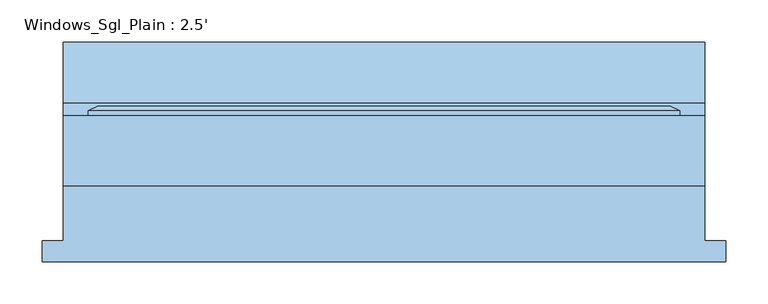
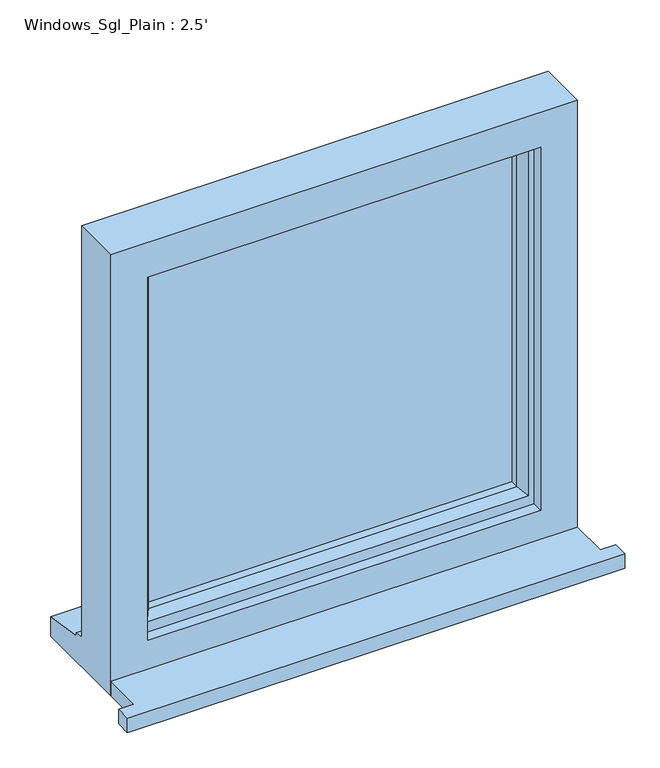
"""IFC4 building model written with IfcOpenShell, lengths in millimetres: window geometry, Windows_Sgl_Plain : 2.5'."""

from ifc_helpers import new_model, si_unit, frame, origin, place, context, project, spatial, polyline, outline, extrude, faceted_brep, source, transform, mapped, element, save


def windows_sgl_plain_2_5_9e76a6e6(model_context):
    return source(origin(), model_context, "Body", "SolidModel", [
        extrude(outline(polyline([(-406.0, -115.6034322), (-406.0, -90.6034322), (-381.0, -90.6034322), (-381.0, -25.4834322), (381.0, -25.4834322), (381.0, -90.6034322), (406.0, -90.6034322), (406.0, -115.6034322), (-406.0, -115.6034322)])), frame((0.0, 0.0, 1348.0), z_axis=(0.0, 0.0, 1.0), x_axis=(1.0, 0.0, 0.0)), (0.0, 0.0, 1.0), 25.0),
        faceted_brep([(-381.0, -25.4834322, 1348.0), (381.0, -25.4834322, 1348.0), (381.0, -25.4834322, 2110.0), (-381.0, -25.4834322, 2110.0), (-321.0, -25.4834322, 2050.0), (321.0, -25.4834322, 2050.0), (321.0, -25.4834322, 1423.0), (-321.0, -25.4834322, 1423.0), (-381.0, 57.5165678, 2110.0), (-381.0, 57.5165678, 1399.0), (-381.0, 72.5165678, 1397.68767), (-381.0, 72.5165678, 1392.7449676), (-381.0, 145.0165678, 1381.8088847), (-381.0, 145.0165678, 1348.0), (381.0, 57.5165678, 2110.0), (381.0, 57.5165678, 1399.0), (-341.0, 57.5165678, 2070.0), (-341.0, 57.5165678, 1411.0), (341.0, 57.5165678, 1411.0), (341.0, 57.5165678, 2070.0), (-341.0, -7.4834322, 2070.0), (-341.0, -7.4834322, 1411.0), (341.0, -7.4834322, 2070.0), (341.0, -7.4834322, 1411.0), (-321.0, -7.4834322, 2050.0), (-321.0, -7.4834322, 1423.0), (321.0, -7.4834322, 1423.0), (321.0, -7.4834322, 2050.0), (381.0, 145.0165678, 1348.0), (381.0, 145.0165678, 1381.8088847), (381.0, 72.5165678, 1392.7449676), (381.0, 72.5165678, 1397.68767)], [[[0, 1, 2, 3], [4, 5, 6, 7]], [[0, 3, 8, 9, 10, 11, 12, 13]], [[9, 8, 14, 15], [16, 17, 18, 19]], [[17, 16, 20, 21]], [[20, 22, 23, 21], [24, 25, 26, 27]], [[24, 4, 7, 25]], [[3, 2, 14, 8]], [[16, 19, 22, 20]], [[5, 4, 24, 27]], [[15, 14, 2, 1, 28, 29, 30, 31]], [[19, 18, 23, 22]], [[5, 27, 26, 6]], [[28, 1, 0, 13]], [[29, 28, 13, 12]], [[30, 29, 12, 11]], [[31, 30, 11, 10]], [[15, 31, 10, 9]], [[21, 23, 18, 17]], [[7, 6, 26, 25]]]),
        extrude(outline(polyline([(311.0, 21.5165678), (-311.0, 21.5165678), (-311.0, 45.5165678), (311.0, 45.5165678), (311.0, 21.5165678)])), frame((0.0, 0.0, 1441.0), z_axis=(0.0, 0.0, 1.0), x_axis=(1.0, 0.0, 0.0)), (0.0, 0.0, 1.0), 599.0),
        faceted_brep([(-351.0, 57.5165678, 2080.0), (-351.0, 63.2900705, 2080.0), (-351.0, 63.2900705, 1401.0), (-351.0, 57.5165678, 1401.0), (-341.0, -7.4834322, 2070.0), (-341.0, 57.5165678, 2070.0), (-341.0, 57.5165678, 1411.0), (-341.0, -7.4834322, 1411.0), (-301.0, 7.0094677, 2030.0), (-311.1480377, -7.4834322, 2040.1480377), (-311.1480377, -7.4834322, 1440.8519623), (-301.0, 7.0094677, 1451.0), (-301.0, 21.5165678, 2030.0), (-301.0, 21.5165678, 1451.0), (-311.0, 45.5165678, 2040.0), (-311.0, 21.5165678, 2040.0), (-311.0, 21.5165678, 1441.0), (-311.0, 45.5165678, 1441.0), (-301.0, 63.2900705, 2030.0), (-301.0, 45.5165678, 2030.0), (-301.0, 45.5165678, 1451.0), (-301.0, 63.2900705, 1451.0), (-318.4457548, 69.0635732, 2047.4457548), (-318.4457548, 69.0635732, 1433.5542452), (-340.2153903, 69.0635732, 2069.2153903), (-340.2153903, 69.0635732, 1411.7846097), (351.0, 63.2900705, 1401.0), (351.0, 57.5165678, 1401.0), (341.0, 57.5165678, 1411.0), (341.0, -7.4834322, 1411.0), (311.1480377, -7.4834322, 1440.8519623), (301.0, 7.0094677, 1451.0), (301.0, 21.5165678, 1451.0), (311.0, 21.5165678, 1441.0), (311.0, 45.5165678, 1441.0), (301.0, 45.5165678, 1451.0), (301.0, 63.2900705, 1451.0), (318.4457548, 69.0635732, 1433.5542452), (340.2153903, 69.0635732, 1411.7846097), (351.0, 63.2900705, 2080.0), (351.0, 57.5165678, 2080.0), (341.0, 57.5165678, 2070.0), (341.0, -7.4834322, 2070.0), (311.1480377, -7.4834322, 2040.1480377), (301.0, 7.0094677, 2030.0), (301.0, 21.5165678, 2030.0), (311.0, 21.5165678, 2040.0), (311.0, 45.5165678, 2040.0), (301.0, 45.5165678, 2030.0), (301.0, 63.2900705, 2030.0), (318.4457548, 69.0635732, 2047.4457548), (340.2153903, 69.0635732, 2069.2153903)], [[[0, 1, 2, 3]], [[4, 5, 6, 7]], [[8, 9, 10, 11]], [[12, 8, 11, 13]], [[14, 15, 16, 17]], [[18, 19, 20, 21]], [[22, 18, 21, 23]], [[1, 24, 25, 2]], [[3, 2, 26, 27]], [[7, 6, 28, 29]], [[11, 10, 30, 31]], [[13, 11, 31, 32]], [[17, 16, 33, 34]], [[21, 20, 35, 36]], [[23, 21, 36, 37]], [[2, 25, 38, 26]], [[27, 26, 39, 40]], [[29, 28, 41, 42]], [[31, 30, 43, 44]], [[32, 31, 44, 45]], [[34, 33, 46, 47]], [[36, 35, 48, 49]], [[37, 36, 49, 50]], [[26, 38, 51, 39]], [[40, 39, 1, 0]], [[3, 27, 40, 0], [5, 41, 28, 6]], [[42, 41, 5, 4]], [[7, 29, 42, 4], [9, 43, 30, 10]], [[44, 43, 9, 8]], [[45, 44, 8, 12]], [[15, 46, 33, 16], [13, 32, 45, 12]], [[47, 46, 15, 14]], [[17, 34, 47, 14], [19, 48, 35, 20]], [[49, 48, 19, 18]], [[50, 49, 18, 22]], [[24, 51, 38, 25], [23, 37, 50, 22]], [[39, 51, 24, 1]]]),
    ])


if __name__ == "__main__":
    model = new_model("IFC4")
    model_context = context("Model", 3, world=origin())
    ifc_project = project(units=[si_unit("LENGTHUNIT", "METRE", prefix="MILLI")], contexts=[model_context])
    site = spatial("IfcSite", under=ifc_project)
    building = spatial("IfcBuilding", under=site)
    placement = place(None, origin())
    windows_sgl_plain_2_5_shape = windows_sgl_plain_2_5_9e76a6e6(model_context)
    element("IfcWindow", 1, ObjectType="Windows_Sgl_Plain : 2.5'", at=placement, inside=building, context=model_context, shape_type="MappedRepresentation", body=[
        mapped(windows_sgl_plain_2_5_shape, transform((0.0, 0.0, 0.0), x_axis=(1.0, 0.0, 0.0), y_axis=(0.0, 1.0, 0.0), z_axis=(0.0, 0.0, 1.0))),
    ])
    save(model, "model.ifc")

# Revit data of these elements
# Type "Windows_Sgl_Plain : 2.5'"
#   Type Mark = "61"
#   Operation = "SinglePanel"
#   Construction Type Id = "SGL"
#   Manufacturer = "Revit"
#   Keynote = "L10"
#   Analytic Construction = "Large single-glazed windows"
#   Wrap Layers (Ext) from Ext = 0.336286 ft
#   Wrap Layers (Int) from Ext = 0.582349 ft
#   Window Board Projection = 0.082021 ft
#   Window Board Extension = 0.082021 ft
#   Visual Light Transmittance = 0.9
#   Solar Heat Gain Coefficient = 0.86
#   Rough Width = 2.5 ft
#   Rough Height = 2.5 ft
#   Height = 2.5 ft
#   Width = 2.5 ft
#   Heat Transfer Coefficient (U) = 5.5617 W/(m²·K)
#   Glazing Thickness = 0.07874 ft
#   FrameOffset - External = 0.164042 ft
#   Frame Depth = 0.213255 ft
#   Default Head Height = 6.922572 ft
#   Cill Depth = 0.287073 ft
#   Cavity Closer Width = 0.164042 ft
#   Cavity Closer Offset from Ext = 0.336286 ft
#   Cavity Closer Depth = 0.278871 ft
#   Vis - Cavity Closers = yes
#   Define Thermal Properties by = 1
#   Material Trim = Window Frame
#   Material Glass = Glass
#   Material Frame = Window Frame
#   Wall Closure = (empty or 0)
# Element 1 (IfcWindow, "Windows_Sgl_Plain : 2.5'")
#   Materials on its faces: "Window Frame", "Glass"
# Materials
#   "Window Frame": colour RGB 249 249 249, transparency 0, Keynote = "L10", Cost = 0
#   "Glass": class "Glass", colour RGB 0 128 192, transparency 0.9, Description = "Soda Lime Glass", Cost = 0
